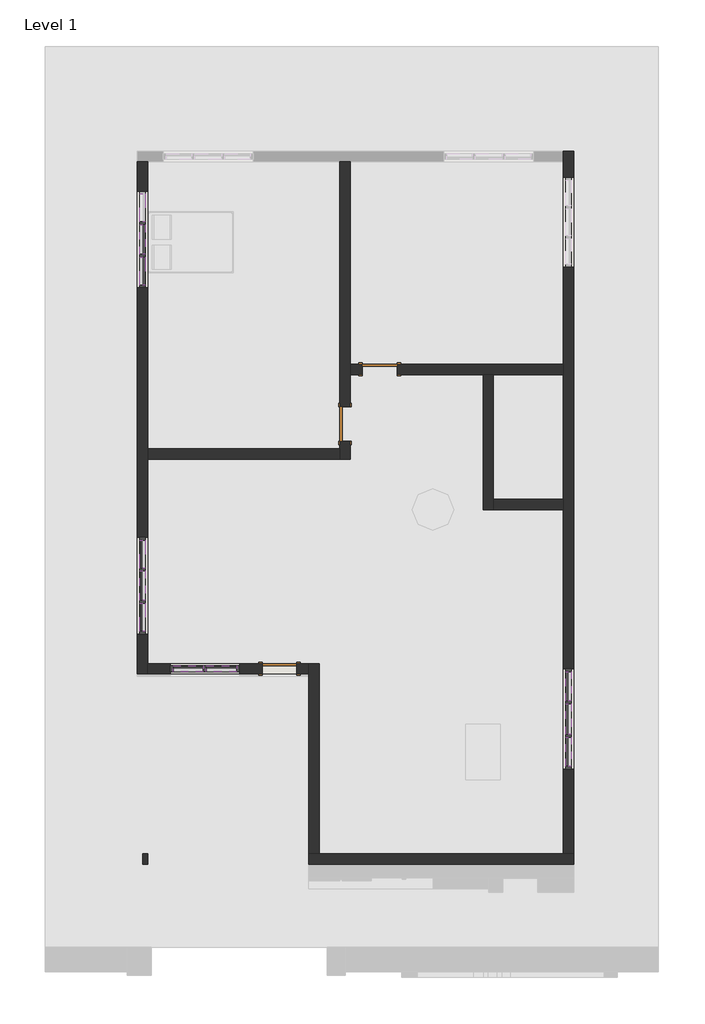
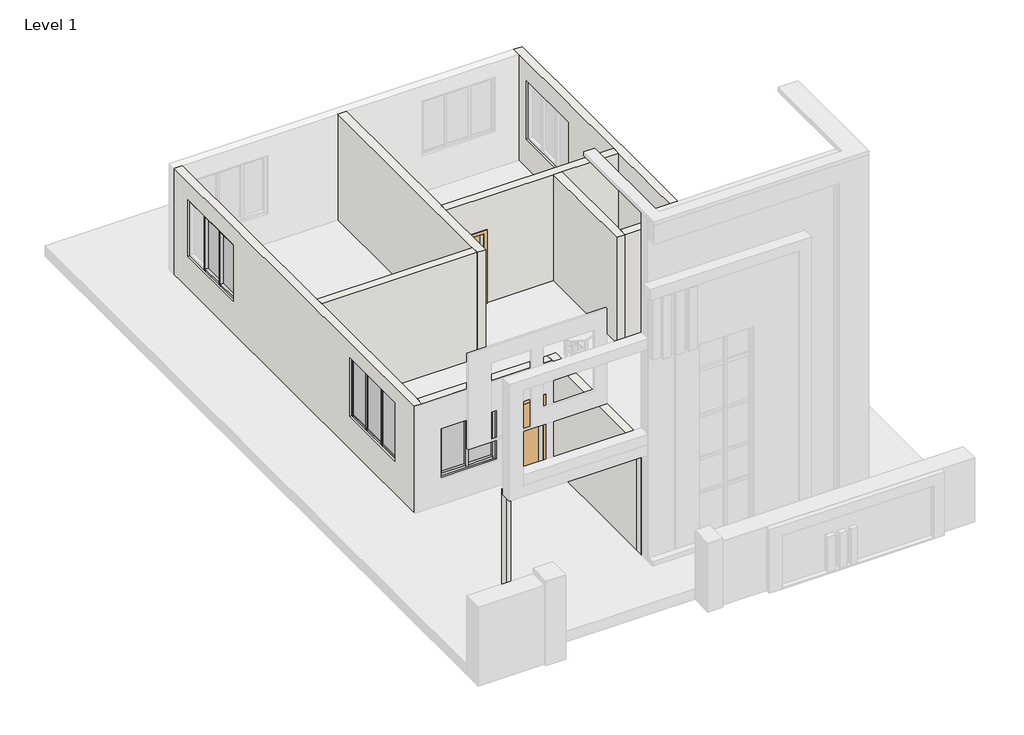
# One storey, part 1 of 2: 35 members, 11 walls, 10 plates, 3 doors.
"""IFC4 building model written with IfcOpenShell, lengths in millimetres."""

from ifc_helpers import new_model, si_unit, frame, origin, origin_with_axes, place, context, project, spatial, polyline, outline, extrude, faceted_brep, transform, mapped, element, save
from components import door_85036156, door_a1484949, member_051277f3, member_dad99500, member_44c1c08d, member_f7325308, member_5215b92c, member_3f0e0172, member_94b81e23, member_8a463cd0, member_e0a154ce, member_4cef4026, member_c33c434a, member_3ae3f724, member_358e2bc9, system_panel_glazed_27fbb1ef, system_panel_glazed_ddf70934, system_panel_glazed_6adbe530, system_panel_glazed_eebfb88d, system_panel_glazed_2519712b, system_panel_glazed_a8f3d8ee, system_panel_glazed_3378ba69

model = new_model("IFC4")

# Units and contexts
model_context = context("Model", 3, world=origin())
ifc_project = project(units=[si_unit("LENGTHUNIT", "METRE", prefix="MILLI")], contexts=[model_context])

# Site, building, storey
site = spatial("IfcSite", under=ifc_project)
building = spatial("IfcBuilding", under=site)
storey = spatial("IfcBuildingStorey", under=building, Name="Level 1", Elevation=0.0)

# Doors
placement = place(None, origin())
door_shape = door_85036156(model_context)
element("IfcDoor", 1, ObjectType="Single-Flush : 30\" x 80\"", at=placement, inside=storey, context=model_context, shape_type="MappedRepresentation", body=[
    mapped(door_shape, transform((-11303.429521, -4650.7001929, 0.0), x_axis=(0.0, -1.0, 0.0), y_axis=(1.0, 0.0, 0.0), z_axis=(0.0, 0.0, 1.0))),
])
element("IfcDoor", 2, ObjectType="Single-Flush : 30\" x 80\"", at=placement, inside=storey, context=model_context, shape_type="MappedRepresentation", body=[
    mapped(door_shape, transform((-10541.429521, -3444.2001929, 0.0), x_axis=(-1.0, 0.0, 0.0), y_axis=(0.0, -1.0, 0.0), z_axis=(0.0, 0.0, 1.0))),
])
door_2_shape = door_a1484949(model_context)
element("IfcDoor", 3, ObjectType="Single-Flush : 30\" x 80\"", at=placement, inside=storey, context=model_context, shape_type="MappedRepresentation", body=[
    mapped(door_2_shape, transform((-12751.229521, -10035.5001929, 50.8), x_axis=(1.0, 0.0, 0.0), y_axis=(0.0, 1.0, 0.0), z_axis=(0.0, 0.0, 1.0))),
])

# Members
member_shape = member_051277f3(model_context)
element("IfcMember", 4, ObjectType="Rectangular Mullion : 2.5\" x 5\" rectangular", at=placement, inside=storey, context=model_context, shape_type="MappedRepresentation", body=[
    mapped(member_shape, transform((-6388.529521, -10803.8501929, 2496.6048955), x_axis=(0.0, 0.0, 1.0), y_axis=(1.0, 0.0, 0.0), z_axis=(0.0, 1.0, 0.0))),
])
member_2_shape = member_dad99500(model_context)
element("IfcMember", 5, ObjectType="Rectangular Mullion : 2.5\" x 5\" rectangular", at=placement, inside=storey, context=model_context, shape_type="MappedRepresentation", body=[
    mapped(member_2_shape, transform((-6388.529521, -11540.4501929, 2496.6048955), x_axis=(0.0, 0.0, 1.0), y_axis=(1.0, 0.0, 0.0), z_axis=(0.0, 1.0, 0.0))),
])
element("IfcMember", 6, ObjectType="Rectangular Mullion : 2.5\" x 5\" rectangular", at=placement, inside=storey, context=model_context, shape_type="MappedRepresentation", body=[
    mapped(member_2_shape, transform((-6388.529521, -10099.0001929, 2496.6048955), x_axis=(0.0, 0.0, 1.0), y_axis=(1.0, 0.0, 0.0), z_axis=(0.0, 1.0, 0.0))),
])
member_3_shape = member_44c1c08d(model_context)
element("IfcMember", 7, ObjectType="Rectangular Mullion : 2.5\" x 5\" rectangular", at=placement, inside=storey, context=model_context, shape_type="MappedRepresentation", body=[
    mapped(member_3_shape, transform((-6388.529521, -10772.1001929, 918.3255169), x_axis=(0.0, 1.0, 0.0), y_axis=(1.0, 0.0, 0.0), z_axis=(0.0, 0.0, -1.0))),
])
element("IfcMember", 8, ObjectType="Rectangular Mullion : 2.5\" x 5\" rectangular", at=placement, inside=storey, context=model_context, shape_type="MappedRepresentation", body=[
    mapped(member_3_shape, transform((-6388.529521, -11508.7001929, 918.3255169), x_axis=(0.0, 1.0, 0.0), y_axis=(1.0, 0.0, 0.0), z_axis=(0.0, 0.0, -1.0))),
])
element("IfcMember", 9, ObjectType="Rectangular Mullion : 2.5\" x 5\" rectangular", at=placement, inside=storey, context=model_context, shape_type="MappedRepresentation", body=[
    mapped(member_2_shape, transform((-6388.529521, -10740.3501929, 918.3255169), x_axis=(0.0, 0.0, -1.0), y_axis=(1.0, 0.0, 0.0), z_axis=(0.0, -1.0, 0.0))),
])
element("IfcMember", 10, ObjectType="Rectangular Mullion : 2.5\" x 5\" rectangular", at=placement, inside=storey, context=model_context, shape_type="MappedRepresentation", body=[
    mapped(member_2_shape, transform((-6388.529521, -12181.8001929, 918.3255169), x_axis=(0.0, 0.0, -1.0), y_axis=(1.0, 0.0, 0.0), z_axis=(0.0, -1.0, 0.0))),
])
element("IfcMember", 11, ObjectType="Rectangular Mullion : 2.5\" x 5\" rectangular", at=placement, inside=storey, context=model_context, shape_type="MappedRepresentation", body=[
    mapped(member_shape, transform((-6388.529521, -11476.9501929, 918.3255169), x_axis=(0.0, 0.0, -1.0), y_axis=(1.0, 0.0, 0.0), z_axis=(0.0, -1.0, 0.0))),
])
member_4_shape = member_f7325308(model_context)
element("IfcMember", 12, ObjectType="Rectangular Mullion : 2.5\" x 5\" rectangular", at=placement, inside=storey, context=model_context, shape_type="MappedRepresentation", body=[
    mapped(member_4_shape, transform((-6388.529521, -10035.5001929, 918.3255169), x_axis=(0.0, 1.0, 0.0), y_axis=(1.0, 0.0, 0.0), z_axis=(0.0, 0.0, -1.0))),
])
element("IfcMember", 13, ObjectType="Rectangular Mullion : 2.5\" x 5\" rectangular", at=placement, inside=storey, context=model_context, shape_type="MappedRepresentation", body=[
    mapped(member_4_shape, transform((-6388.529521, -12245.3001929, 2496.6048955), x_axis=(0.0, -1.0, 0.0), y_axis=(1.0, 0.0, 0.0), z_axis=(0.0, 0.0, 1.0))),
])
member_5_shape = member_5215b92c(model_context)
element("IfcMember", 14, ObjectType="Rectangular Mullion : 2.5\" x 5\" rectangular", at=placement, inside=storey, context=model_context, shape_type="MappedRepresentation", body=[
    mapped(member_5_shape, transform((-15761.129521, -910.5501929, 2533.943824), x_axis=(0.0, 0.0, 1.0), y_axis=(-1.0, 0.0, 0.0), z_axis=(0.0, -1.0, 0.0))),
])
element("IfcMember", 15, ObjectType="Rectangular Mullion : 2.5\" x 5\" rectangular", at=placement, inside=storey, context=model_context, shape_type="MappedRepresentation", body=[
    mapped(member_5_shape, transform((-15761.129521, -7882.8501929, 2626.593654), x_axis=(0.0, 0.0, 1.0), y_axis=(1.0, 0.0, 0.0), z_axis=(0.0, 1.0, 0.0))),
])
member_6_shape = member_3f0e0172(model_context)
element("IfcMember", 16, ObjectType="Rectangular Mullion : 2.5\" x 5\" rectangular", at=placement, inside=storey, context=model_context, shape_type="MappedRepresentation", body=[
    mapped(member_6_shape, transform((-15761.129521, -199.3501929, 2533.943824), x_axis=(0.0, 0.0, 1.0), y_axis=(-1.0, 0.0, 0.0), z_axis=(0.0, -1.0, 0.0))),
])
element("IfcMember", 17, ObjectType="Rectangular Mullion : 2.5\" x 5\" rectangular", at=placement, inside=storey, context=model_context, shape_type="MappedRepresentation", body=[
    mapped(member_6_shape, transform((-15761.129521, -1590.0001929, 2533.943824), x_axis=(0.0, 0.0, 1.0), y_axis=(-1.0, 0.0, 0.0), z_axis=(0.0, -1.0, 0.0))),
])
element("IfcMember", 18, ObjectType="Rectangular Mullion : 2.5\" x 5\" rectangular", at=placement, inside=storey, context=model_context, shape_type="MappedRepresentation", body=[
    mapped(member_6_shape, transform((-15761.129521, -8594.0501929, 2626.593654), x_axis=(0.0, 0.0, 1.0), y_axis=(1.0, 0.0, 0.0), z_axis=(0.0, 1.0, 0.0))),
])
element("IfcMember", 19, ObjectType="Rectangular Mullion : 2.5\" x 5\" rectangular", at=placement, inside=storey, context=model_context, shape_type="MappedRepresentation", body=[
    mapped(member_6_shape, transform((-15761.129521, -7203.4001929, 2626.593654), x_axis=(0.0, 0.0, 1.0), y_axis=(1.0, 0.0, 0.0), z_axis=(0.0, 1.0, 0.0))),
])
member_7_shape = member_94b81e23(model_context)
element("IfcMember", 20, ObjectType="Rectangular Mullion : 2.5\" x 5\" rectangular", at=placement, inside=storey, context=model_context, shape_type="MappedRepresentation", body=[
    mapped(member_7_shape, transform((-15761.129521, -231.1001929, 913.1300213), x_axis=(0.0, -1.0, 0.0), y_axis=(-1.0, 0.0, 0.0), z_axis=(0.0, 0.0, -1.0))),
])
element("IfcMember", 21, ObjectType="Rectangular Mullion : 2.5\" x 5\" rectangular", at=placement, inside=storey, context=model_context, shape_type="MappedRepresentation", body=[
    mapped(member_7_shape, transform((-15761.129521, -942.3001929, 913.1300213), x_axis=(0.0, -1.0, 0.0), y_axis=(-1.0, 0.0, 0.0), z_axis=(0.0, 0.0, -1.0))),
])
element("IfcMember", 22, ObjectType="Rectangular Mullion : 2.5\" x 5\" rectangular", at=placement, inside=storey, context=model_context, shape_type="MappedRepresentation", body=[
    mapped(member_6_shape, transform((-15761.129521, -974.0501929, 913.1300213), x_axis=(0.0, 0.0, -1.0), y_axis=(-1.0, 0.0, 0.0), z_axis=(0.0, 1.0, 0.0))),
])
element("IfcMember", 23, ObjectType="Rectangular Mullion : 2.5\" x 5\" rectangular", at=placement, inside=storey, context=model_context, shape_type="MappedRepresentation", body=[
    mapped(member_6_shape, transform((-15761.129521, -7819.3501929, 939.496743), x_axis=(0.0, 0.0, -1.0), y_axis=(1.0, 0.0, 0.0), z_axis=(0.0, -1.0, 0.0))),
])
element("IfcMember", 24, ObjectType="Rectangular Mullion : 2.5\" x 5\" rectangular", at=placement, inside=storey, context=model_context, shape_type="MappedRepresentation", body=[
    mapped(member_6_shape, transform((-15761.129521, -9210.0001929, 939.496743), x_axis=(0.0, 0.0, -1.0), y_axis=(1.0, 0.0, 0.0), z_axis=(0.0, -1.0, 0.0))),
])
element("IfcMember", 25, ObjectType="Rectangular Mullion : 2.5\" x 5\" rectangular", at=placement, inside=storey, context=model_context, shape_type="MappedRepresentation", body=[
    mapped(member_5_shape, transform((-15761.129521, -262.8501929, 913.1300213), x_axis=(0.0, 0.0, -1.0), y_axis=(-1.0, 0.0, 0.0), z_axis=(0.0, 1.0, 0.0))),
])
element("IfcMember", 26, ObjectType="Rectangular Mullion : 2.5\" x 5\" rectangular", at=placement, inside=storey, context=model_context, shape_type="MappedRepresentation", body=[
    mapped(member_5_shape, transform((-15761.129521, -8530.5501929, 939.496743), x_axis=(0.0, 0.0, -1.0), y_axis=(1.0, 0.0, 0.0), z_axis=(0.0, -1.0, 0.0))),
])
member_8_shape = member_8a463cd0(model_context)
element("IfcMember", 27, ObjectType="Rectangular Mullion : 2.5\" x 5\" rectangular", at=placement, inside=storey, context=model_context, shape_type="MappedRepresentation", body=[
    mapped(member_8_shape, transform((-15761.129521, -1653.5001929, 913.1300213), x_axis=(0.0, -1.0, 0.0), y_axis=(-1.0, 0.0, 0.0), z_axis=(0.0, 0.0, -1.0))),
])
member_9_shape = member_e0a154ce(model_context)
element("IfcMember", 28, ObjectType="Rectangular Mullion : 2.5\" x 5\" rectangular", at=placement, inside=storey, context=model_context, shape_type="MappedRepresentation", body=[
    mapped(member_9_shape, transform((-15761.129521, -7851.1001929, 939.496743), x_axis=(0.0, 1.0, 0.0), y_axis=(1.0, 0.0, 0.0), z_axis=(0.0, 0.0, -1.0))),
])
element("IfcMember", 29, ObjectType="Rectangular Mullion : 2.5\" x 5\" rectangular", at=placement, inside=storey, context=model_context, shape_type="MappedRepresentation", body=[
    mapped(member_9_shape, transform((-15761.129521, -8562.3001929, 939.496743), x_axis=(0.0, 1.0, 0.0), y_axis=(1.0, 0.0, 0.0), z_axis=(0.0, 0.0, -1.0))),
])
member_10_shape = member_4cef4026(model_context)
element("IfcMember", 30, ObjectType="Rectangular Mullion : 2.5\" x 5\" rectangular", at=placement, inside=storey, context=model_context, shape_type="MappedRepresentation", body=[
    mapped(member_10_shape, transform((-15761.129521, -9273.5001929, 2626.593654), x_axis=(0.0, -1.0, 0.0), y_axis=(1.0, 0.0, 0.0), z_axis=(0.0, 0.0, 1.0))),
])
element("IfcMember", 31, ObjectType="Rectangular Mullion : 2.5\" x 5\" rectangular", at=placement, inside=storey, context=model_context, shape_type="MappedRepresentation", body=[
    mapped(member_10_shape, transform((-15761.129521, -7139.9001929, 939.496743), x_axis=(0.0, 1.0, 0.0), y_axis=(1.0, 0.0, 0.0), z_axis=(0.0, 0.0, -1.0))),
])
member_11_shape = member_c33c434a(model_context)
element("IfcMember", 32, ObjectType="Rectangular Mullion : 2.5\" x 5\" rectangular", at=placement, inside=storey, context=model_context, shape_type="MappedRepresentation", body=[
    mapped(member_11_shape, transform((-14421.279521, -10035.5001929, 2181.7525261), x_axis=(0.0, 0.0, 1.0), y_axis=(0.0, -1.0, 0.0), z_axis=(1.0, 0.0, 0.0))),
])
element("IfcMember", 33, ObjectType="Rectangular Mullion : 2.5\" x 5\" rectangular", at=placement, inside=storey, context=model_context, shape_type="MappedRepresentation", body=[
    mapped(member_11_shape, transform((-13691.029521, -10035.5001929, 2181.7525261), x_axis=(0.0, 0.0, 1.0), y_axis=(0.0, -1.0, 0.0), z_axis=(1.0, 0.0, 0.0))),
])
member_12_shape = member_3ae3f724(model_context)
element("IfcMember", 34, ObjectType="Rectangular Mullion : 2.5\" x 5\" rectangular", at=placement, inside=storey, context=model_context, shape_type="MappedRepresentation", body=[
    mapped(member_12_shape, transform((-14389.529521, -10035.5001929, 750.5784943), x_axis=(1.0, 0.0, 0.0), y_axis=(0.0, -1.0, 0.0), z_axis=(0.0, 0.0, -1.0))),
])
element("IfcMember", 35, ObjectType="Rectangular Mullion : 2.5\" x 5\" rectangular", at=placement, inside=storey, context=model_context, shape_type="MappedRepresentation", body=[
    mapped(member_11_shape, transform((-14357.779521, -10035.5001929, 750.5784943), x_axis=(0.0, 0.0, -1.0), y_axis=(0.0, -1.0, 0.0), z_axis=(-1.0, 0.0, 0.0))),
])
element("IfcMember", 36, ObjectType="Rectangular Mullion : 2.5\" x 5\" rectangular", at=placement, inside=storey, context=model_context, shape_type="MappedRepresentation", body=[
    mapped(member_11_shape, transform((-15088.029521, -10035.5001929, 750.5784943), x_axis=(0.0, 0.0, -1.0), y_axis=(0.0, -1.0, 0.0), z_axis=(-1.0, 0.0, 0.0))),
])
member_13_shape = member_358e2bc9(model_context)
element("IfcMember", 37, ObjectType="Rectangular Mullion : 2.5\" x 5\" rectangular", at=placement, inside=storey, context=model_context, shape_type="MappedRepresentation", body=[
    mapped(member_13_shape, transform((-13627.529521, -10035.5001929, 750.5784943), x_axis=(1.0, 0.0, 0.0), y_axis=(0.0, -1.0, 0.0), z_axis=(0.0, 0.0, -1.0))),
])
element("IfcMember", 38, ObjectType="Rectangular Mullion : 2.5\" x 5\" rectangular", at=placement, inside=storey, context=model_context, shape_type="MappedRepresentation", body=[
    mapped(member_13_shape, transform((-15151.529521, -10035.5001929, 2181.7525261), x_axis=(-1.0, 0.0, 0.0), y_axis=(0.0, -1.0, 0.0), z_axis=(0.0, 0.0, 1.0))),
])

# Plates
system_panel_glazed_shape = system_panel_glazed_27fbb1ef(model_context)
element("IfcPlate", 39, ObjectType="System Panel : Glazed", at=placement, inside=storey, context=model_context, shape_type="MappedRepresentation", body=[
    mapped(system_panel_glazed_shape, transform((-6388.529521, -11140.4001929, 981.8255169), x_axis=(0.0, 1.0, 0.0), y_axis=(-1.0, 0.0, 0.0), z_axis=(0.0, 0.0, 1.0))),
])
system_panel_glazed_2_shape = system_panel_glazed_ddf70934(model_context)
element("IfcPlate", 40, ObjectType="System Panel : Glazed", at=placement, inside=storey, context=model_context, shape_type="MappedRepresentation", body=[
    mapped(system_panel_glazed_2_shape, transform((-6388.529521, -11861.1251929, 981.8255169), x_axis=(0.0, 1.0, 0.0), y_axis=(-1.0, 0.0, 0.0), z_axis=(0.0, 0.0, 1.0))),
])
element("IfcPlate", 41, ObjectType="System Panel : Glazed", at=placement, inside=storey, context=model_context, shape_type="MappedRepresentation", body=[
    mapped(system_panel_glazed_2_shape, transform((-6388.529521, -10419.6751929, 981.8255169), x_axis=(0.0, 1.0, 0.0), y_axis=(-1.0, 0.0, 0.0), z_axis=(0.0, 0.0, 1.0))),
])
system_panel_glazed_3_shape = system_panel_glazed_6adbe530(model_context)
element("IfcPlate", 42, ObjectType="System Panel : Glazed", at=placement, inside=storey, context=model_context, shape_type="MappedRepresentation", body=[
    mapped(system_panel_glazed_3_shape, transform((-15761.129521, -586.7001929, 976.6300213), x_axis=(0.0, -1.0, 0.0), y_axis=(1.0, 0.0, 0.0), z_axis=(0.0, 0.0, 1.0))),
])
system_panel_glazed_4_shape = system_panel_glazed_eebfb88d(model_context)
element("IfcPlate", 43, ObjectType="System Panel : Glazed", at=placement, inside=storey, context=model_context, shape_type="MappedRepresentation", body=[
    mapped(system_panel_glazed_4_shape, transform((-15761.129521, -1282.0251929, 976.6300213), x_axis=(0.0, -1.0, 0.0), y_axis=(1.0, 0.0, 0.0), z_axis=(0.0, 0.0, 1.0))),
])
system_panel_glazed_5_shape = system_panel_glazed_2519712b(model_context)
element("IfcPlate", 44, ObjectType="System Panel : Glazed", at=placement, inside=storey, context=model_context, shape_type="MappedRepresentation", body=[
    mapped(system_panel_glazed_5_shape, transform((-15761.129521, -8902.0251929, 1002.996743), x_axis=(0.0, 1.0, 0.0), y_axis=(-1.0, 0.0, 0.0), z_axis=(0.0, 0.0, 1.0))),
])
element("IfcPlate", 45, ObjectType="System Panel : Glazed", at=placement, inside=storey, context=model_context, shape_type="MappedRepresentation", body=[
    mapped(system_panel_glazed_5_shape, transform((-15761.129521, -7511.3751929, 1002.996743), x_axis=(0.0, 1.0, 0.0), y_axis=(-1.0, 0.0, 0.0), z_axis=(0.0, 0.0, 1.0))),
])
system_panel_glazed_6_shape = system_panel_glazed_a8f3d8ee(model_context)
element("IfcPlate", 46, ObjectType="System Panel : Glazed", at=placement, inside=storey, context=model_context, shape_type="MappedRepresentation", body=[
    mapped(system_panel_glazed_6_shape, transform((-15761.129521, -8206.7001929, 1002.996743), x_axis=(0.0, 1.0, 0.0), y_axis=(-1.0, 0.0, 0.0), z_axis=(0.0, 0.0, 1.0))),
])
system_panel_glazed_7_shape = system_panel_glazed_3378ba69(model_context)
element("IfcPlate", 47, ObjectType="System Panel : Glazed", at=placement, inside=storey, context=model_context, shape_type="MappedRepresentation", body=[
    mapped(system_panel_glazed_7_shape, transform((-14754.654521, -10035.5001929, 814.0784943), x_axis=(1.0, 0.0, 0.0), y_axis=(0.0, 1.0, 0.0), z_axis=(0.0, 0.0, 1.0))),
])
element("IfcPlate", 48, ObjectType="System Panel : Glazed", at=placement, inside=storey, context=model_context, shape_type="MappedRepresentation", body=[
    mapped(system_panel_glazed_7_shape, transform((-14024.404521, -10035.5001929, 814.0784943), x_axis=(1.0, 0.0, 0.0), y_axis=(0.0, 1.0, 0.0), z_axis=(0.0, 0.0, 1.0))),
])

# Walls
element("IfcWall", 49, ObjectType="9\"", at=placement, inside=storey, context=model_context, shape_type="SweptSolid", body=[
    extrude(outline(polyline([(-15646.829521, -14340.8001929), (-15761.129521, -14340.8001929), (-15761.129521, -14112.2001929), (-15646.829521, -14112.2001929), (-15646.829521, -14340.8001929)])), origin_with_axes(), (0.0, 0.0, 1.0), 3048.0),
])
element("IfcWall", 50, ObjectType="9\"", at=placement, inside=storey, context=model_context, shape_type="Brep", body=[
    faceted_brep([(-6274.229521, -14112.2001929, 0.0), (-6274.229521, 1356.3998071, 0.0), (-6274.229521, 1356.3998071, 3048.0), (-6274.229521, -14112.2001929, 3048.0), (-6274.229521, -12245.3001929, 918.3255169), (-6274.229521, -12245.3001929, 2496.6048955), (-6274.229521, -10035.5001929, 2496.6048955), (-6274.229521, -10035.5001929, 918.3255169), (-6274.229521, 784.8998071, 2498.2989313), (-6274.229521, 784.8998071, 812.0853055), (-6274.229521, -1196.3001929, 812.0853055), (-6274.229521, -1196.3001929, 2498.2989313), (-6502.829521, 1356.3998071, 0.0), (-6502.829521, 1127.7998071, 0.0), (-6502.829521, -3329.9001929, 0.0), (-6502.829521, -3558.5001929, 0.0), (-6502.829521, -6301.7001929, 0.0), (-6502.829521, -6530.3001929, 0.0), (-6502.829521, -14112.2001929, 0.0), (-6502.829521, -14112.2001929, 3048.0), (-6502.829521, -6530.3001929, 3048.0), (-6502.829521, -6301.7001929, 3048.0), (-6502.829521, -3558.5001929, 3048.0), (-6502.829521, -3329.9001929, 3048.0), (-6502.829521, 1127.7998071, 3048.0), (-6502.829521, 1356.3998071, 3048.0), (-6502.829521, -12245.3001929, 2496.6048955), (-6502.829521, -12245.3001929, 918.3255169), (-6502.829521, -10035.5001929, 918.3255169), (-6502.829521, -10035.5001929, 2496.6048955), (-6502.829521, 784.8998071, 812.0853055), (-6502.829521, 784.8998071, 2498.2989313), (-6502.829521, -1196.3001929, 2498.2989313), (-6502.829521, -1196.3001929, 812.0853055)], [[[0, 1, 2, 3], [4, 5, 6, 7], [8, 9, 10, 11]], [[12, 13, 14, 15, 16, 17, 18, 19, 20, 21, 22, 23, 24, 25], [26, 27, 28, 29], [30, 31, 32, 33]], [[1, 0, 18, 17, 16, 15, 14, 13, 12]], [[3, 2, 25, 24, 23, 22, 21, 20, 19]], [[0, 3, 19, 18]], [[2, 1, 12, 25]], [[26, 5, 4, 27]], [[5, 26, 29, 6]], [[6, 29, 28, 7]], [[27, 4, 7, 28]], [[30, 9, 8, 31]], [[31, 8, 11, 32]], [[32, 11, 10, 33]], [[9, 30, 33, 10]]]),
])
element("IfcWall", 51, ObjectType="9\"", at=placement, inside=storey, context=model_context, shape_type="Brep", body=[
    faceted_brep([(-15875.429521, 1127.7998071, 0.0), (-15875.429521, -10149.8001929, 0.0), (-15875.429521, -10149.8001929, 3048.0), (-15875.429521, 1127.7998071, 3048.0), (-15875.429521, 480.0998071, 913.1300213), (-15875.429521, 480.0998071, 2533.943824), (-15875.429521, -1653.5001929, 2533.943824), (-15875.429521, -1653.5001929, 913.1300213), (-15875.429521, -9273.5001929, 2626.593654), (-15875.429521, -9273.5001929, 939.496743), (-15875.429521, -7139.9001929, 939.496743), (-15875.429521, -7139.9001929, 2626.593654), (-15646.829521, -10149.8001929, 0.0), (-15646.829521, -9921.2001929, 0.0), (-15646.829521, -5425.4001929, 0.0), (-15646.829521, -5196.8001929, 0.0), (-15646.829521, 1127.7998071, 0.0), (-15646.829521, 1127.7998071, 3048.0), (-15646.829521, -5196.8001929, 3048.0), (-15646.829521, -5425.4001929, 3048.0), (-15646.829521, -9921.2001929, 3048.0), (-15646.829521, -10149.8001929, 3048.0), (-15646.829521, 480.0998071, 2533.943824), (-15646.829521, 480.0998071, 913.1300213), (-15646.829521, -1653.5001929, 913.1300213), (-15646.829521, -1653.5001929, 2533.943824), (-15646.829521, -9273.5001929, 939.496743), (-15646.829521, -9273.5001929, 2626.593654), (-15646.829521, -7139.9001929, 2626.593654), (-15646.829521, -7139.9001929, 939.496743)], [[[0, 1, 2, 3], [4, 5, 6, 7], [8, 9, 10, 11]], [[12, 13, 14, 15, 16, 17, 18, 19, 20, 21], [22, 23, 24, 25], [26, 27, 28, 29]], [[1, 0, 16, 15, 14, 13, 12]], [[2, 1, 12, 21]], [[3, 2, 21, 20, 19, 18, 17]], [[0, 3, 17, 16]], [[4, 23, 22, 5]], [[5, 22, 25, 6]], [[6, 25, 24, 7]], [[23, 4, 7, 24]], [[26, 9, 8, 27]], [[27, 8, 11, 28]], [[10, 29, 28, 11]], [[9, 26, 29, 10]]]),
])
element("IfcWall", 52, ObjectType="9\"", at=placement, inside=storey, context=model_context, shape_type="Brep", body=[
    faceted_brep([(-11874.929521, -14112.2001929, 0.0), (-11874.929521, -9921.2001929, 0.0), (-11874.929521, -9921.2001929, 3048.0), (-11874.929521, -14112.2001929, 3048.0), (-12103.529521, -14112.2001929, 0.0), (-12103.529521, -14112.2001929, 3048.0), (-12103.529521, -10149.8001929, 3048.0), (-12103.529521, -9921.2001929, 3048.0), (-12103.529521, -9921.2001929, 0.0), (-12103.529521, -10149.8001929, 0.0)], [[[0, 1, 2, 3]], [[4, 5, 6, 7, 8, 9]], [[1, 0, 4, 9, 8]], [[3, 2, 7, 6, 5]], [[0, 3, 5, 4]], [[2, 1, 8, 7]]]),
])
element("IfcWall", 53, ObjectType="9\"", at=placement, inside=storey, context=model_context, shape_type="SweptSolid", body=[
    extrude(outline(polyline([(0.0, -15646.829521), (0.0, -12103.529521), (3048.0, -12103.529521), (3048.0, -15646.829521), (0.0, -15646.829521)]), holes=[polyline([(50.8, -12370.229521), (50.8, -13132.229521), (2082.8, -13132.229521), (2082.8, -12370.229521), (50.8, -12370.229521)]), polyline([(750.5784943, -15151.529521), (2181.7525261, -15151.529521), (2181.7525261, -13627.529521), (750.5784943, -13627.529521), (750.5784943, -15151.529521)])]), frame((0.0, -10149.8001929, 0.0), z_axis=(0.0, 1.0, 0.0), x_axis=(0.0, 0.0, 1.0)), (0.0, 0.0, 1.0), 228.6),
])
element("IfcWall", 54, ObjectType="9\"", at=placement, inside=storey, context=model_context, shape_type="Brep", body=[
    faceted_brep([(-11417.729521, -5031.7001929, 2032.0), (-11417.729521, -5031.7001929, 0.0), (-11417.729521, -5196.8001929, 0.0), (-11417.729521, -5425.4001929, 0.0), (-11417.729521, -5425.4001929, 3048.0), (-11417.729521, -5196.8001929, 3048.0), (-11417.729521, 1127.7998071, 3048.0), (-11417.729521, 1127.7998071, 0.0), (-11417.729521, -4269.7001929, 0.0), (-11417.729521, -4269.7001929, 2032.0), (-11189.129521, -5425.4001929, 0.0), (-11189.129521, -5031.7001929, 0.0), (-11189.129521, -5031.7001929, 2032.0), (-11189.129521, -4269.7001929, 2032.0), (-11189.129521, -4269.7001929, 0.0), (-11189.129521, -3558.5001929, 0.0), (-11189.129521, -3329.9001929, 0.0), (-11189.129521, 1127.7998071, 0.0), (-11189.129521, 1127.7998071, 3048.0), (-11189.129521, -3329.9001929, 3048.0), (-11189.129521, -3558.5001929, 3048.0), (-11189.129521, -5425.4001929, 3048.0)], [[[0, 1, 2, 3, 4, 5, 6, 7, 8, 9]], [[10, 11, 12, 13, 14, 15, 16, 17, 18, 19, 20, 21]], [[8, 7, 17, 16, 15, 14]], [[3, 2, 1, 11, 10]], [[6, 5, 4, 21, 20, 19, 18]], [[7, 6, 18, 17]], [[4, 3, 10, 21]], [[12, 11, 1, 0]], [[13, 12, 0, 9]], [[14, 13, 9, 8]]]),
])
element("IfcWall", 55, ObjectType="9\"", at=placement, inside=storey, context=model_context, shape_type="SweptSolid", body=[
    extrude(outline(polyline([(-15646.829521, -5196.8001929), (-11417.729521, -5196.8001929), (-11417.729521, -5425.4001929), (-15646.829521, -5425.4001929), (-15646.829521, -5196.8001929)])), origin_with_axes(), (0.0, 0.0, 1.0), 3048.0),
])
element("IfcWall", 56, ObjectType="9\"", at=placement, inside=storey, context=model_context, shape_type="Brep", body=[
    faceted_brep([(-11189.129521, -3558.5001929, 0.0), (-10922.429521, -3558.5001929, 0.0), (-10922.429521, -3558.5001929, 2032.0), (-10160.429521, -3558.5001929, 2032.0), (-10160.429521, -3558.5001929, 0.0), (-8268.129521, -3558.5001929, 0.0), (-8039.529521, -3558.5001929, 0.0), (-6502.829521, -3558.5001929, 0.0), (-6502.829521, -3558.5001929, 3048.0), (-8039.529521, -3558.5001929, 3048.0), (-8268.129521, -3558.5001929, 3048.0), (-11189.129521, -3558.5001929, 3048.0), (-10922.429521, -3329.9001929, 2032.0), (-10922.429521, -3329.9001929, 0.0), (-11189.129521, -3329.9001929, 0.0), (-11189.129521, -3329.9001929, 3048.0), (-6502.829521, -3329.9001929, 3048.0), (-6502.829521, -3329.9001929, 0.0), (-10160.429521, -3329.9001929, 0.0), (-10160.429521, -3329.9001929, 2032.0)], [[[0, 1, 2, 3, 4, 5, 6, 7, 8, 9, 10, 11]], [[12, 13, 14, 15, 16, 17, 18, 19]], [[18, 17, 7, 6, 5, 4]], [[14, 13, 1, 0]], [[11, 10, 9, 8, 16, 15]], [[8, 7, 17, 16]], [[0, 11, 15, 14]], [[2, 1, 13, 12]], [[3, 2, 12, 19]], [[4, 3, 19, 18]]]),
])
element("IfcWall", 57, ObjectType="9\"", at=placement, inside=storey, context=model_context, shape_type="Brep", body=[
    faceted_brep([(-8268.129521, -3558.5001929, 0.0), (-8268.129521, -6530.3001929, 0.0), (-8268.129521, -6530.3001929, 3048.0), (-8268.129521, -3558.5001929, 3048.0), (-8039.529521, -3558.5001929, 0.0), (-8039.529521, -3558.5001929, 3048.0), (-8039.529521, -6301.7001929, 3048.0), (-8039.529521, -6530.3001929, 3048.0), (-8039.529521, -6530.3001929, 0.0), (-8039.529521, -6301.7001929, 0.0)], [[[0, 1, 2, 3]], [[4, 5, 6, 7, 8, 9]], [[1, 0, 4, 9, 8]], [[3, 2, 7, 6, 5]], [[0, 3, 5, 4]], [[2, 1, 8, 7]]]),
])
element("IfcWall", 58, ObjectType="9\"", at=placement, inside=storey, context=model_context, shape_type="SweptSolid", body=[
    extrude(outline(polyline([(-6502.829521, -6530.3001929), (-8039.529521, -6530.3001929), (-8039.529521, -6301.7001929), (-6502.829521, -6301.7001929), (-6502.829521, -6530.3001929)])), origin_with_axes(), (0.0, 0.0, 1.0), 3048.0),
])
element("IfcWall", 59, ObjectType="9\"", at=placement, inside=storey, context=model_context, shape_type="Brep", body=[
    faceted_brep([(-12103.529521, -14340.8001929, 0.0), (-6274.229521, -14340.8001929, 0.0), (-6274.229521, -14340.8001929, 3048.0), (-12103.529521, -14340.8001929, 3048.0), (-12103.529521, -14112.2001929, 0.0), (-12103.529521, -14112.2001929, 3048.0), (-11874.929521, -14112.2001929, 3048.0), (-6502.829521, -14112.2001929, 3048.0), (-6274.229521, -14112.2001929, 3048.0), (-6274.229521, -14112.2001929, 0.0), (-6502.829521, -14112.2001929, 0.0), (-11874.929521, -14112.2001929, 0.0)], [[[0, 1, 2, 3]], [[4, 5, 6, 7, 8, 9, 10, 11]], [[1, 0, 4, 11, 10, 9]], [[3, 2, 8, 7, 6, 5]], [[0, 3, 5, 4]], [[2, 1, 9, 8]]]),
])

save(model, "model.ifc")

# Revit data of these elements
# Type "Single-Flush : 30\" x 80\""
#   Type Mark = "5"
#   Construction Type Id = "MDOOR"
#   Assembly Code = "C1020"
#   Analytic Construction = "Metal"
#   Thickness = 0' - 2"
#   Heat Transfer Coefficient (U) = 0.651978 BTU/(h·ft²·°F)
#   Height = 6' - 8"
#   Trim Projection Ext = 0' - 1"
#   Trim Projection Int = 0' - 1"
#   Trim Width = 0' - 3"
#   Width = 2' - 6"
#   Define Thermal Properties by = 1
#   Define Thermal Properties by = 1
#   Door Material = Door - Panel
#   Frame Material = Door - Frame
#   Visual Light Transmittance = 0
#   Solar Heat Gain Coefficient = 0
#   Function = (empty or 0)
#   Wall Closure = (empty or 0)
# Type "Rectangular Mullion : 2.5\" x 5\" rectangular"
#   built-in parameter 1007304 = 0.416667 (stored number, unit not read)
#   built-in parameter 1007301 = 0.104167 (stored number, unit not read)
#   built-in parameter 1007300 = 0.104167 (stored number, unit not read)
# Type "System Panel : Glazed"
#   Construction Type Id = "GSP4R"
#   Analytic Construction = "1/8 in Pilkington single glazing"
#   Visual Light Transmittance = 0.9
#   Solar Heat Gain Coefficient = 0.86
#   Heat Transfer Coefficient (U) = 1.18115 BTU/(h·ft²·°F)
#   Define Thermal Properties by = 1
# Type "9\""
#   Assembly Code = "B2010"
#   Layers, outside or top first: 0' - 9" no material (function 1)
# Elements 1, 2, 3 (IfcDoor, "Single-Flush : 30\" x 80\"")
#   Phase Created = New Construction
#   Materials on its faces: "Door - Frame", "Door - Panel"
# Elements 4, 5, 6, 7, 8, 9, 10, 11, 12, 13, 14, 15, 16, 17, 18, 19, 20, 21, 22, 23, 24, 25, 26, 27, 28, 29, 30, 31, 32, 33, 34, 35, 36, 37, 38 (IfcMember, "Rectangular Mullion : 2.5\" x 5\" rectangular")
#   Phase Created = New Construction
#   Materials on its faces: "Aluminum"
# Elements 39, 40, 41, 42, 43, 44, 45, 46, 47, 48 (IfcPlate, "System Panel : Glazed")
#   Phase Created = New Construction
#   Materials on its faces: "Glass"
# Elements 49, 50, 51, 52, 53, 54, 55, 56, 57, 58, 59 (IfcWall, "9\"")
#   Top Offset = 0' - 0"
#   Base Offset = 0' - 0"
#   Unconnected Height = 10' - 0"
#   wall height = 10' - 0"
#   Phase Created = New Construction
#   Base Constraint = Level 1
#   Materials on its faces: "Default Wall"
# Materials
#   "Door - Panel": class "Wood", colour RGB 210 159 95, transparency 0, Cost = 0
#   "Door - Frame": colour RGB 118 70 51, transparency 0, Cost = 0
#   "Aluminum": class "Metal", colour RGB 247 247 247, transparency 0, Description = "Aluminum 6061", Cost = 0
#   "Glass": class "Glass", colour RGB 0 128 192, transparency 0.75, Description = "Soda Lime Glass", Cost = 0
#   "Default Wall": colour RGB 128 128 128, transparency 0, Cost = 0
